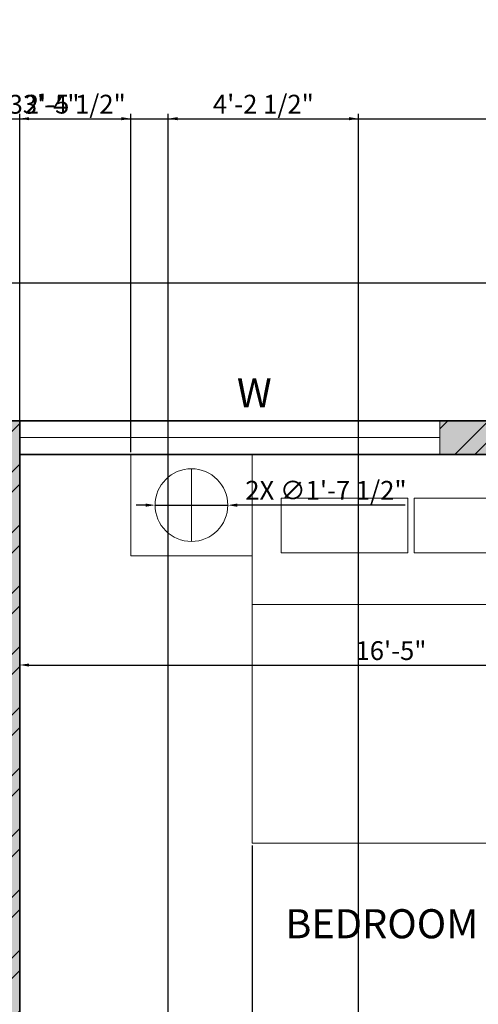
# Model space of a CAD drawing. Units: inches. Extents: x 1804 to 3296, y 909 to 2477.
# Tile 19 of 31: x 2119 to 2241, y 1638 to 1900. Entities that reach past the tile are written whole.
import ezdxf

# ---------------------------------------------------------------- set-up
doc = ezdxf.new("R2010")
doc.units = ezdxf.units.IN
for name, color, linetype, lineweight in [('A-ANNO-DIMS', 2, 'Continuous', 18), ('A-ANNO-TTLB', 156, 'Continuous', 35), ('A-AREA-IDEN', 190, 'Continuous', 18), ('A-WALL-PATT', 10, 'Continuous', 13), ('C-PROP', 7, 'Continuous', 25), ('FUR', 100, 'Continuous', 18), ('TEXT', 190, 'Continuous', 18), ('WALL', 10, 'Continuous', 35), ('WIND', 130, 'Continuous', 18)]:
    doc.layers.add(name, color=color, linetype=linetype, lineweight=lineweight)
doc.styles.get("Standard").update_dxf_attribs({"font": 'arial.ttf'})
doc.dimstyles.new('ISO-25', dxfattribs={"dimtxt": 5, "dimasz": 2.5, "dimexe": 1.25, "dimexo": 0.625, "dimtad": 1, "dimdec": 0, "dimlunit": 4, "dimtxsty": 'Standard', "dimcen": 2.5, "dimadec": 0, "dimazin": 0, "dimtfac": 1, "dimtdec": 0, "dimtmove": 0, "dimatfit": 3, "dimfxl": 1, "dimarcsym": 0})
pattern_1 = [(45, (0, 196.207), (-8.08223, 8.08223), []), (45, (5.388, 196.207), (-8.08223, 8.08223), [])]

# ---------------------------------------------------------------- blocks, each defined once
blk = doc.blocks.new('*D10')
at = {"layer": 'A-ANNO-DIMS', "color": 0, "lineweight": -2, "transparency": 16777216}
for p, q in [((2119.08, 1783.75), (2119.08, 1727.15)), ((2316.54, 1783.75), (2316.54, 1727.15)), ((2121.58, 1728.4), (2314.04, 1728.4))]:
    blk.add_line(p, q, dxfattribs=at)
at = {"layer": 'A-ANNO-DIMS', "color": 0, "lineweight": 100, "transparency": 16777216}
for points in [[(2121.58, 1728.81), (2121.58, 1727.98), (2119.08, 1728.4)], [(2314.04, 1728.81), (2314.04, 1727.98), (2316.54, 1728.4)]]:
    blk.add_solid(points, dxfattribs=at)
at = {"layer": 'Defpoints', "color": 0, "lineweight": 100, "transparency": 16777216}
for p in [(2119.08, 1784.38), (2316.54, 1784.38), (2316.54, 1728.4)]:
    blk.add_point(p, dxfattribs=at)
at = {"layer": 'A-ANNO-DIMS', "color": 0, "transparency": 16777216, "insert": (2217.81, 1731.58), "char_height": 5, "attachment_point": 5}
blk.add_mtext('16\'-5"', dxfattribs=at)
blk = doc.blocks.new('WINDOW-PLAN-112IN')
blk.add_line((0, 4.5), (111.7, 4.5))
blk.add_lwpolyline([(0, 0), (111.7, 0), (111.7, 9), (0, 9)], close=True)
blk = doc.blocks.new('NIGHTSTAND-WITH-LAMP')
for p, q in [((16.12, 3.78), (16.12, 23.13)), ((6.45, 13.46), (25.79, 13.46))]:
    blk.add_line(p, q)
blk.add_lwpolyline([(32.24, 26.91), (0, 26.91), (0, 0), (32.24, 0)], close=True)
blk.add_circle((16.12, 13.46), 9.67)
blk = doc.blocks.new('*D51')
at = {"layer": 'A-ANNO-DIMS', "color": 0, "lineweight": -2, "transparency": 16777216}
for p, q in [((1925.58, 1830.66), (1925.58, 1874.99)), ((1928.08, 1873.74), (2323.04, 1873.74)), ((2325.54, 1830.66), (2325.54, 1874.99))]:
    blk.add_line(p, q, dxfattribs=at)
at = {"layer": 'A-ANNO-DIMS', "color": 0, "lineweight": 100, "transparency": 16777216}
for points in [[(1928.08, 1874.15), (1928.08, 1873.32), (1925.58, 1873.74)], [(2323.04, 1874.15), (2323.04, 1873.32), (2325.54, 1873.74)]]:
    blk.add_solid(points, dxfattribs=at)
at = {"layer": 'Defpoints', "color": 0, "lineweight": 100, "transparency": 16777216}
for p in [(2325.54, 1873.74), (1925.58, 1830.04), (2325.54, 1830.04)]:
    blk.add_point(p, dxfattribs=at)
at = {"layer": 'A-ANNO-DIMS', "color": 0, "transparency": 16777216, "insert": (2125.56, 1876.92), "char_height": 5, "attachment_point": 5}
blk.add_mtext('33\'-4"', dxfattribs=at)
blk = doc.blocks.new('*D56')
at = {"layer": 'A-ANNO-DIMS', "color": 0, "lineweight": -2, "transparency": 16777216}
for p, q in [((2180.87, 1680.42), (2180.87, 975.89)), ((2268, 1680.42), (2268, 975.89)), ((2183.37, 977.14), (2265.5, 977.14))]:
    blk.add_line(p, q, dxfattribs=at)
at = {"layer": 'A-ANNO-DIMS', "color": 0, "lineweight": 100, "transparency": 16777216}
for points in [[(2183.37, 977.56), (2183.37, 976.72), (2180.87, 977.14)], [(2265.5, 977.56), (2265.5, 976.72), (2268, 977.14)]]:
    blk.add_solid(points, dxfattribs=at)
at = {"layer": 'Defpoints', "color": 0, "lineweight": 100, "transparency": 16777216}
for p in [(2180.87, 1681.04), (2268, 1681.04), (2268, 977.14)]:
    blk.add_point(p, dxfattribs=at)
at = {"layer": 'A-ANNO-DIMS', "color": 0, "transparency": 16777216, "insert": (2224.44, 980.32), "char_height": 5, "attachment_point": 5}
blk.add_mtext('7\'-3"', dxfattribs=at)
blk = doc.blocks.new('*D58')
at = {"layer": 'A-ANNO-DIMS', "color": 0, "lineweight": -2, "transparency": 16777216}
for p, q in [((2119.08, 1785), (2119.08, 1874.99)), ((2121.58, 1873.74), (2146.13, 1873.74)), ((2148.63, 1785), (2148.63, 1874.99))]:
    blk.add_line(p, q, dxfattribs=at)
at = {"layer": 'A-ANNO-DIMS', "color": 0, "lineweight": 100, "transparency": 16777216}
for points in [[(2121.58, 1874.15), (2121.58, 1873.32), (2119.08, 1873.74)], [(2146.13, 1874.15), (2146.13, 1873.32), (2148.63, 1873.74)]]:
    blk.add_solid(points, dxfattribs=at)
at = {"layer": 'Defpoints', "color": 0, "lineweight": 100, "transparency": 16777216}
for p in [(2148.63, 1873.74), (2119.08, 1784.38), (2148.63, 1784.38)]:
    blk.add_point(p, dxfattribs=at)
at = {"layer": 'A-ANNO-DIMS', "color": 0, "transparency": 16777216, "insert": (2133.86, 1876.95), "char_height": 5, "attachment_point": 5}
blk.add_mtext('2\'-5 1/2"', dxfattribs=at)
blk = doc.blocks.new('*D71')
at = {"layer": 'A-ANNO-DIMS', "color": 0, "lineweight": -2, "transparency": 16777216}
for p, q in [((2158.58, 1272.26), (2158.58, 1874.99)), ((2161.08, 1873.74), (2206.69, 1873.74)), ((2209.19, 1272.26), (2209.19, 1874.99))]:
    blk.add_line(p, q, dxfattribs=at)
at = {"layer": 'A-ANNO-DIMS', "color": 0, "lineweight": 100, "transparency": 16777216}
for points in [[(2161.08, 1874.15), (2161.08, 1873.32), (2158.58, 1873.74)], [(2206.69, 1874.15), (2206.69, 1873.32), (2209.19, 1873.74)]]:
    blk.add_solid(points, dxfattribs=at)
at = {"layer": 'Defpoints', "color": 0, "lineweight": 100, "transparency": 16777216}
for p in [(2209.19, 1873.74), (2158.58, 1271.63), (2209.19, 1271.63)]:
    blk.add_point(p, dxfattribs=at)
at = {"layer": 'A-ANNO-DIMS', "color": 0, "transparency": 16777216, "insert": (2183.88, 1876.95), "char_height": 5, "attachment_point": 5}
blk.add_mtext('4\'-2 1/2"', dxfattribs=at)
blk = doc.blocks.new('*D102')
at = {"layer": 'A-ANNO-DIMS', "color": 0, "lineweight": -2, "transparency": 16777216}
for p, q in [((2152.58, 1770.93), (2150.08, 1770.93)), ((2155.08, 1770.93), (2174.42, 1770.92)), ((2221.62, 1770.9), (2176.92, 1770.92))]:
    blk.add_line(p, q, dxfattribs=at)
at = {"layer": 'A-ANNO-DIMS', "color": 0, "lineweight": 100, "transparency": 16777216}
for points in [[(2152.58, 1771.35), (2152.58, 1770.51), (2155.08, 1770.93)], [(2176.92, 1771.34), (2176.92, 1770.5), (2174.42, 1770.92)]]:
    blk.add_solid(points, dxfattribs=at)
at = {"layer": 'Defpoints', "color": 0, "lineweight": 100, "transparency": 16777216}
for p in [(2155.08, 1770.93), (2174.42, 1770.92)]:
    blk.add_point(p, dxfattribs=at)
at = {"layer": 'A-ANNO-DIMS', "color": 0, "transparency": 16777216, "insert": (2200.52, 1774.23), "char_height": 5, "attachment_point": 5, "rotation": 359.9776}
blk.add_mtext('2X ∅1\'-7 1/2"', dxfattribs=at)

msp = doc.modelspace()

# ---------------------------------------------------------------- hatches: boundary and pattern name
at = {"layer": 'A-ANNO-TTLB'}
h = msp.add_hatch(color=256, dxfattribs=at)
h.dxf.hatch_style = 1
h.paths.add_polyline_path([(3294.53, 2476.54), (1803.79, 2476.54), (1805.43, 909.47), (3296.17, 909.47)])
h.paths.add_polyline_path([(1811, 914.33), (1812.79, 2467.54), (3285.53, 2467.54), (3283.74, 914.33)], flags=16)
h.paths.add_polyline_path([(1925.58, 1062.77), (1925.58, 1138.07), (1925.58, 1539.88), (1925.58, 1793.38), (1925.58, 1830.04), (2325.54, 1830.04), (2325.54, 1793.38), (2325.54, 1586.42), (2325.54, 1138.07), (2325.54, 1062.77)], flags=0)
h.paths.add_polyline_path([(1997.22, 1029.4), (2008.85, 1037.96), (2008.85, 1020.84)], flags=0)
h.paths.add_polyline_path([(1934.58, 1138.07), (1934.58, 1147.07), (2078.77, 1147.07), (2078.77, 1138.07), (2060.94, 1138.07)], flags=0)
h.paths.add_polyline_path([(1944.35, 1138.07), (1944.35, 1147.07), (2056.05, 1147.07), (2056.05, 1138.07)], flags=0)
h.paths.add_polyline_path([(2222.24, 1037.96), (2233.87, 1029.4), (2222.24, 1020.84)], flags=0)
h.paths.add_polyline_path([(2061.94, 1139.07), (2061.94, 1146.07), (2077.77, 1146.07), (2077.77, 1139.07)], flags=0)
h.paths.add_polyline_path([(2149.58, 1138.07), (2149.58, 1269.44), (2158.58, 1269.44), (2158.58, 1326.69), (2149.58, 1326.69), (2149.58, 1340.94), (2139.6, 1340.94), (2139.6, 1434.25), (2149.58, 1434.25), (2149.58, 1447.36), (2158.58, 1447.36), (2158.58, 1423.87), (2158.58, 1408.06), (2198.46, 1408.06), (2198.46, 1412.56), (2282.65, 1412.56), (2282.65, 1465.94), (2316.54, 1465.94), (2316.54, 1590.92), (2192.86, 1590.92), (2192.86, 1595.3), (2291.17, 1595.3), (2291.17, 1590.92), (2316.54, 1590.92), (2316.54, 1784.38), (2300.24, 1784.38), (2300.24, 1757.47), (2268, 1757.47), (2268, 1681.04), (2180.87, 1681.04), (2180.87, 1757.47), (2148.63, 1757.47), (2148.63, 1784.38), (2119.08, 1784.38), (2119.08, 1585.58), (2114.58, 1585.58), (2114.58, 1784.38), (2064.11, 1784.38), (2046.28, 1784.38), (2046.28, 1760.38), (1958.58, 1760.38), (1958.58, 1664.38), (1934.58, 1664.38), (1934.58, 1784.38), (1934.58, 1793.38), (2046.28, 1793.38), (2064.11, 1793.38), (2119.08, 1793.38), (2230.78, 1793.38), (2230.78, 1784.38), (2268, 1784.38), (2300.24, 1784.38), (2316.54, 1784.38), (2316.54, 1590.92), (2316.54, 1373.73), (2316.54, 1138.07)], flags=0)
h.paths.add_polyline_path([(2209.19, 1166.63), (2209.19, 1175.63), (2158.58, 1175.63), (2209.19, 1223.63), (2209.19, 1231.63), (2183.88, 1231.63), (2183.88, 1301.66), (2242.59, 1301.66), (2242.59, 1326.69), (2316.54, 1326.69), (2272.59, 1271.63), (2272.59, 1223.63), (2316.54, 1175.63), (2272.59, 1175.63), (2272.59, 1166.63)], flags=0)
h.paths.add_polyline_path([(1947.77, 1345.22), (1947.77, 1457.48), (1991.2, 1457.48), (1991.2, 1451.7), (1991.2, 1352.18), (1991.2, 1345.22)], flags=0)
h.paths.add_polyline_path([(2209.19, 1271.63), (2262.59, 1271.63), (2262.59, 1311.85), (2272.59, 1301.66), (2272.59, 1271.63), (2269.92, 1269.63), (2270.59, 1269.63), (2270.59, 1225.63), (2211.19, 1225.63), (2211.19, 1269.63), (2211.86, 1269.63)], flags=0)
h.paths.add_polyline_path([(2000.34, 1378.21), (2000.34, 1429.71), (2025.22, 1429.71), (2025.22, 1378.21)], flags=0)
h.paths.add_polyline_path([(2001.34, 1379.21), (2001.34, 1428.71), (2024.22, 1428.71), (2024.22, 1379.21)], flags=0)
h.paths.add_polyline_path([(2012.34, 1390.21), (2012.34, 1417.71), (2013.22, 1417.71), (2013.22, 1390.21)], flags=0)
h.paths.add_polyline_path([(2237.56, 1331.19), (2237.56, 1340.18), (2238.62, 1340.18), (2238.62, 1386.84), (2241.04, 1386.84), (2242.06, 1386.84), (2242.06, 1408.06), (2316.54, 1331.19)], flags=0)
h.paths.add_polyline_path([(1953.73, 1464.35), (1953.73, 1498.59), (1981.74, 1498.59), (1981.74, 1464.35)], flags=0)
h.paths.add_polyline_path([(1987.63, 1462.08), (1987.63, 1500.95), (2104.07, 1500.95), (2104.07, 1462.08), (2099.27, 1462.08), (1993.6, 1462.08)], flags=0)
h.paths.add_polyline_path([(1956.06, 1481.47, -1), (1979.41, 1481.47, -1)], flags=0)
edge = h.paths.add_edge_path(flags=0)
edge.add_ellipse((2299.53, 1438.37), major_axis=(0.31, 21.36), ratio=0.670333, start_angle=0, end_angle=360)
h.paths.add_polyline_path([(2297.39, 1438.37, -1), (2301.67, 1438.37, -1)], flags=0)
h.paths.add_polyline_path([(2591.54, 1163.23), (2591.54, 1179.38), (2591.54, 1379.68), (2591.54, 1395.84), (2734.5, 1395.84), (2734.5, 1379.68), (2734.5, 1179.38), (2734.5, 1163.23)], flags=0)
h.paths.add_polyline_path([(2592.54, 1164.23), (2592.54, 1166.23), (2733.5, 1166.23), (2733.5, 1164.23)], flags=0)
h.paths.add_polyline_path([(2592.54, 1180.38), (2592.54, 1378.68), (2733.5, 1378.68), (2733.5, 1180.38)], flags=0)
h.paths.add_polyline_path([(2593.54, 1181.38), (2593.54, 1377.68), (2732.5, 1377.68), (2732.5, 1181.38)], flags=0)
h.paths.add_polyline_path([(2594.54, 1182.38), (2594.54, 1376.68), (2731.5, 1376.68), (2731.5, 1182.38)], flags=0)
h.paths.add_polyline_path([(1936.95, 1697.46), (1936.95, 1736.46), (1955.41, 1736.46), (1955.41, 1697.46)], flags=0)
h.paths.add_polyline_path([(1938.48, 1718.36), (1938.48, 1734.92), (1953.65, 1734.92), (1953.65, 1718.36)], flags=0)
h.paths.add_polyline_path([(1944.75, 1726.64, -1), (1947.37, 1726.64, -1)], flags=0)
h.paths.add_polyline_path([(2592.54, 1394.84), (2733.5, 1394.84), (2733.5, 1392.84), (2592.54, 1392.84)], flags=0)
h.paths.add_polyline_path([(1976.61, 1762.5), (1976.61, 1781.44), (2012.79, 1781.44), (2012.79, 1762.5)], flags=0)
h.paths.add_polyline_path([(1979.57, 1771.97, -1), (1991.39, 1771.97, -1)], flags=0)
h.paths.add_polyline_path([(1995.36, 1771.97, -1), (2007.18, 1771.97, -1)], flags=0)
h.paths.add_polyline_path([(2251.51, 1744.53), (2268, 1730.05), (2251.51, 1730.05)], flags=0)
h.paths.add_polyline_path([(2047.28, 1785.38), (2047.28, 1792.38), (2063.11, 1792.38), (2063.11, 1785.38)], flags=0)
h.paths.add_polyline_path([(2155.08, 1770.92, -1), (2174.42, 1770.92, -1)], flags=0)
h.paths.add_polyline_path([(2188.59, 1758.27), (2188.59, 1772.81), (2222.3, 1772.81), (2222.3, 1758.27)], flags=0)
h.paths.add_polyline_path([(2223.97, 1758.27), (2223.97, 1772.81), (2257.68, 1772.81), (2257.68, 1758.27)], flags=0)
h.paths.add_polyline_path([(2274.45, 1770.92, -1), (2293.8, 1770.92, -1)], flags=0)
h.paths.add_polyline_path([(2591.54, 1582.09), (2591.54, 1782.39), (2734.5, 1782.39), (2734.5, 1582.09)], flags=0)
h.paths.add_polyline_path([(2592.54, 1583.09), (2592.54, 1781.39), (2733.5, 1781.39), (2733.5, 1583.09)], flags=0)
h.paths.add_polyline_path([(2593.54, 1584.09), (2593.54, 1780.39), (2732.5, 1780.39), (2732.5, 1584.09)], flags=0)
h.paths.add_polyline_path([(2594.54, 1585.09), (2594.54, 1779.39), (2731.5, 1779.39), (2731.5, 1585.09)], flags=0)
h.paths.add_polyline_path([(1922.17, 1978.79), (1922.17, 2295.08), (1922.17, 2296.08), (2115.67, 2296.08), (2115.67, 2384.31), (2115.67, 2385.31), (2322.12, 2385.31), (2323.12, 2385.31), (2323.12, 1979.79), (2323.12, 1978.79), (1923.17, 1978.79)], flags=0)
h.paths.add_polyline_path([(1922.17, 1978.79), (1922.17, 2051.31), (1922.17, 2214.86), (1922.17, 2296.08), (2115.67, 2296.08), (2115.67, 2385.31), (2323.12, 2385.31), (2323.12, 2280.42), (2323.12, 1978.79), (2115.67, 1978.79)], flags=0)
h.paths.add_polyline_path([(1923.17, 1979.79), (1923.17, 2050.31), (2115.67, 2050.31), (2115.67, 2051.31), (1923.17, 2051.31), (1923.17, 2213.86), (1923.17, 2214.86), (1923.17, 2295.08), (1990.02, 2295.08), (1990.02, 2214.86), (1991.02, 2214.86), (1991.02, 2295.08), (2115.67, 2295.08), (2115.67, 1979.79), (2116.67, 1979.79), (2116.67, 2304.18), (2116.67, 2384.31), (2322.12, 2384.31), (2322.12, 2280.42), (2322.12, 1979.79), (2115.67, 1979.79)], flags=0)
h.paths.add_polyline_path([(2972.46, 1192.5), (2972.46, 1196.92), (2995.47, 1196.92), (2995.47, 1255.47), (2995.09, 1255.47), (2987.42, 1249.39), (2980.08, 1255.47), (2978.05, 1255.47), (2978.05, 1257.24), (2995.47, 1257.24), (2995.47, 1261.58), (3015.37, 1261.58), (3015.37, 1333.28), (3015.37, 1414.4), (3032.82, 1414.4), (3032.82, 1333.28), (3032.82, 1261.58), (3052.66, 1261.58), (3052.66, 1255.47), (3079.86, 1255.47), (3078.72, 1254.57), (3081.47, 1252.29), (3078.56, 1249.99), (3075.81, 1252.26), (3072.57, 1249.69), (3070.36, 1251.52), (3067.67, 1249.39), (3060.34, 1255.47), (3052.66, 1255.47), (3052.66, 1196.92), (3054.58, 1196.92), (3074, 1196.92), (3074, 1192.5), (3052.66, 1192.5), (2995.47, 1192.5)], flags=0)
h.paths.add_polyline_path([(2490.75, 1979.27), (2490.75, 1980.27), (2596.87, 1980.27), (2596.87, 2051.8), (2596.87, 2052.8), (2596.87, 2216.35), (2596.87, 2297.57), (2717.32, 2297.57), (2710.57, 2305.62), (2724.07, 2305.62), (2717.32, 2297.57), (2782.37, 2297.57), (2782.37, 2395.8), (3006.82, 2395.8), (3006.82, 1981.27), (3093.73, 1981.27), (3093.73, 1980.27), (3047.51, 1980.27), (3046.37, 1979.37), (3049.11, 1977.1), (3046.2, 1974.79), (3043.46, 1977.07), (3040.21, 1974.49), (3038, 1976.32), (3035.32, 1974.2), (3027.98, 1980.27), (2871.83, 1980.27), (2871.83, 1981.27), (2791.37, 1981.27), (2791.37, 2050.8), (2597.87, 2050.8), (2597.87, 1980.27), (2597.87, 1979.27), (2546.27, 1979.27), (2545.12, 1978.37), (2547.87, 1976.1), (2544.96, 1973.79), (2542.22, 1976.07), (2538.97, 1973.49), (2536.76, 1975.32), (2534.07, 1973.2), (2526.74, 1979.27)], flags=0)
h.paths.add_polyline_path([(2597.87, 2051.8), (2606.87, 2051.8), (2606.87, 2258.39), (2597.87, 2258.39), (2597.87, 2296.57), (2606.87, 2296.57), (2606.87, 2262.39), (2782.37, 2262.39), (2782.37, 2296.57), (2790.37, 2296.57), (2790.37, 2262.39), (2791.37, 2262.39), (2791.37, 2305.67), (2791.37, 2385.8), (2996.82, 2385.8), (2996.82, 2339.85), (3006.82, 2339.85), (3006.82, 2250.12), (2997.82, 2250.12), (2997.82, 1981.27), (2996.82, 1981.27), (2872.83, 1981.27), (2872.83, 1991.8), (2871.83, 1991.8), (2871.83, 2050.8), (2790.37, 2050.8), (2597.87, 2050.8)], flags=0)
h.paths.add_polyline_path([(2179.93, 2153.92), (2179.93, 2353.97), (2259.98, 2353.97), (2259.98, 2153.92)], flags=0)
h.paths.add_polyline_path([(2180.93, 2154.92), (2180.93, 2352.97), (2258.98, 2352.97), (2258.98, 2154.92)], flags=0)
h.paths.add_polyline_path([(2960.87, 1608.49), (2960.87, 1753.62), (3070.9, 1753.62), (3070.9, 1608.49)], flags=0)
h.paths.add_polyline_path([(2961.87, 1609.49), (2961.87, 1752.62), (3069.9, 1752.62), (3069.9, 1609.49)], flags=0)
h.paths.add_polyline_path([(2962.87, 1610.49), (2962.87, 1751.62), (3068.9, 1751.62), (3068.9, 1610.49)], flags=0)
h.paths.add_polyline_path([(2963.87, 1611.49), (2963.87, 1750.62), (3067.9, 1750.62), (3067.9, 1611.49)], flags=0)
h.paths.add_polyline_path([(2782.37, 2051.8), (2782.37, 2216.32), (2791.37, 2216.32), (2791.37, 2051.8), (2872.83, 2051.8), (2872.83, 2068.56), (2884.67, 2068.56), (2884.67, 2085.33), (2896.51, 2085.33), (2896.51, 2102.09), (2908.36, 2102.09), (2908.36, 2118.85), (2920.2, 2118.85), (2920.2, 2135.62), (2932.05, 2135.62), (2932.05, 2145.3), (2925.08, 2145.3), (2925.08, 2203.2), (2996.82, 2203.2), (2996.82, 2145.3), (2953.82, 2145.3), (2872.83, 2051.8), (2790.37, 2051.8)], flags=0)
h.paths.add_polyline_path([(2717.32, 2238.65), (2710.57, 2246.7), (2724.07, 2246.7)], flags=0)
h.paths.add_polyline_path([(2003.09, 1122.79), (2017.16, 1122.79), (2017.16, 1138.74), (2003.09, 1138.74)], flags=8)
h.paths.add_polyline_path([(2174.76, 1792.72), (2188.83, 1792.72), (2188.83, 1808.66), (2174.76, 1808.66)], flags=8)
h.paths.add_polyline_path([(1987.95, 1792.51), (2002.02, 1792.51), (2002.02, 1808.45), (1987.95, 1808.45)], flags=8)
h.paths.add_polyline_path([(2148.79, 1289.26), (2160.46, 1289.26), (2160.46, 1305.2), (2148.79, 1305.2)], flags=8)
h.paths.add_polyline_path([(2115.36, 1133.57), (2127.04, 1133.57), (2127.04, 1149.51), (2115.36, 1149.51)], flags=8)
h.paths.add_polyline_path([(2237.58, 1421.48), (2249.25, 1421.48), (2249.25, 1437.43), (2237.58, 1437.43)], flags=8)
h.paths.add_polyline_path([(2134.99, 1584.32), (2146.66, 1584.32), (2146.66, 1600.26), (2134.99, 1600.26)], flags=8)
h.paths.add_polyline_path([(2101.95, 1557.31), (2113.62, 1557.31), (2113.62, 1573.25), (2101.95, 1573.25)], flags=8)
h.paths.add_polyline_path([(2937.85, 1156.77), (3120.41, 1156.77), (3120.41, 1185.72), (2937.85, 1185.72)], flags=8)
h.paths.add_polyline_path([(2980.71, 1786.71), (3050.06, 1786.71), (3050.06, 1802.66), (2980.71, 1802.66)], flags=8)
h.paths.add_polyline_path([(2869.28, 1661.96), (2938.62, 1661.96), (2938.62, 1690.8), (2869.28, 1690.8)], flags=8)
h.paths.add_polyline_path([(3092.27, 1674.86), (3161.62, 1674.86), (3161.62, 1690.8), (3092.27, 1690.8)], flags=8)
h.paths.add_polyline_path([(2980.71, 1674.86), (3050.06, 1674.86), (3050.06, 1690.8), (2980.71, 1690.8)], flags=8)
h.paths.add_polyline_path([(2649.07, 1678.23), (2674.53, 1678.23), (2674.53, 1714.76), (2649.07, 1714.76)], flags=8)
h.paths.add_polyline_path([(2530.84, 1981.63), (2549.13, 1981.63), (2549.13, 1997.57), (2530.84, 1997.57)], flags=8)
h.paths.add_polyline_path([(3031.29, 1981.77), (3049.58, 1981.77), (3049.58, 1997.71), (3031.29, 1997.71)], flags=8)
h.paths.add_polyline_path([(2715.38, 1911.9), (2851.54, 1911.9), (2851.54, 1940.85), (2715.38, 1940.85)], flags=8)
h.paths.add_polyline_path([(2015.23, 1927.36), (2205.42, 1927.36), (2205.42, 1956.3), (2015.23, 1956.3)], flags=8)
h.paths.add_polyline_path([(2671.84, 2057.84), (2702.75, 2057.84), (2702.75, 2073.79), (2671.84, 2073.79)], flags=8)
h.paths.add_polyline_path([(2678.5, 2316.52), (2765.26, 2316.52), (2765.26, 2332.46), (2678.5, 2332.46)], flags=8)
h.paths.add_polyline_path([(2678.48, 2271.96), (2736.41, 2271.96), (2736.41, 2287.9), (2678.48, 2287.9)], flags=8)
h.paths.add_polyline_path([(2019.2, 972.79), (2243.21, 972.79), (2243.21, 1001.74), (2019.2, 1001.74)], flags=8)
h.paths.add_polyline_path([(2097.06, 1021.56), (2132.16, 1021.56), (2132.16, 1037.51), (2097.06, 1037.51)], flags=8)
h.paths.add_polyline_path([(2182.47, 1360.48), (2207.35, 1360.48), (2207.35, 1376.42), (2182.47, 1376.42)], flags=8)
h.paths.add_polyline_path([(2261.12, 1361.77), (2295.01, 1361.77), (2295.01, 1377.71), (2261.12, 1377.71)], flags=8)
h.paths.add_polyline_path([(2245.75, 1511.51), (2278.44, 1511.51), (2278.44, 1527.46), (2245.75, 1527.46)], flags=8)
h.paths.add_polyline_path([(1991.16, 1296.29), (2060.51, 1296.29), (2060.51, 1312.23), (1991.16, 1312.23)], flags=8)
h.paths.add_polyline_path([(2187, 1651.35), (2246.71, 1651.35), (2246.71, 1667.29), (2187, 1667.29)], flags=8)
h.paths.add_polyline_path([(1976.49, 1684.81), (2068.63, 1684.81), (2068.63, 1700.76), (1976.49, 1700.76)], flags=8)
at = {"layer": 'A-WALL-PATT'}
h = msp.add_hatch(color=256, dxfattribs=at)
h.dxf.hatch_style = 1
h.paths.add_polyline_path([(2119.08, 1544.38), (1925.58, 1544.38), (1925.58, 1539.88), (2119.08, 1539.88)])
h.paths.add_polyline_path([(2119.08, 1545.58), (2114.58, 1545.58), (2114.58, 1544.38), (2119.08, 1544.38)])
h.paths.add_polyline_path([(1965.87, 1658.79), (1965.87, 1679.09), (1955.57, 1679.09), (1955.57, 1658.79)], flags=9)
h.paths.add_polyline_path([(2293.18, 1677.29), (2293.18, 1697.58), (2282.88, 1697.58), (2282.88, 1677.29)], flags=9)
h.paths.add_polyline_path([(2271.13, 1545.23), (2287.53, 1545.23), (2287.53, 1555.53), (2271.13, 1555.53)], flags=9)
h.paths.add_polyline_path([(2303.26, 1488.52), (2303.26, 1508.82), (2292.95, 1508.82), (2292.95, 1488.52)], flags=9)
h.paths.add_polyline_path([(2271.13, 1393.15), (2287.53, 1393.15), (2287.53, 1403.45), (2271.13, 1403.45)], flags=9)
h.paths.add_polyline_path([(2306.48, 1361.45), (2306.48, 1377.86), (2296.18, 1377.86), (2296.18, 1361.45)], flags=9)
h.paths.add_polyline_path([(2174.54, 1361.45), (2174.54, 1377.86), (2164.23, 1377.86), (2164.23, 1361.45)], flags=9)
h.paths.add_polyline_path([(1968.21, 1333.34), (1968.21, 1353.64), (1957.91, 1353.64), (1957.91, 1333.34)], flags=9)
h.paths.add_polyline_path([(2003.09, 1122.79), (2017.16, 1122.79), (2017.16, 1138.74), (2003.09, 1138.74)], flags=9)
h.paths.add_polyline_path([(2174.76, 1792.72), (2188.83, 1792.72), (2188.83, 1808.66), (2174.76, 1808.66)], flags=9)
h.paths.add_polyline_path([(1987.95, 1792.51), (2002.02, 1792.51), (2002.02, 1808.45), (1987.95, 1808.45)], flags=9)
h.paths.add_polyline_path([(2148.79, 1289.26), (2160.46, 1289.26), (2160.46, 1305.2), (2148.79, 1305.2)], flags=9)
h.paths.add_polyline_path([(2115.36, 1133.57), (2127.04, 1133.57), (2127.04, 1149.51), (2115.36, 1149.51)], flags=9)
h.paths.add_polyline_path([(2237.58, 1421.48), (2249.25, 1421.48), (2249.25, 1437.43), (2237.58, 1437.43)], flags=9)
h.paths.add_polyline_path([(2134.99, 1584.32), (2146.66, 1584.32), (2146.66, 1600.26), (2134.99, 1600.26)], flags=9)
h.paths.add_polyline_path([(2101.95, 1557.31), (2113.62, 1557.31), (2113.62, 1573.25), (2101.95, 1573.25)], flags=9)
h.paths.add_polyline_path([(2937.85, 1156.77), (3120.41, 1156.77), (3120.41, 1185.72), (2937.85, 1185.72)], flags=9)
h.paths.add_polyline_path([(2980.71, 1786.71), (3050.06, 1786.71), (3050.06, 1802.66), (2980.71, 1802.66)], flags=9)
h.paths.add_polyline_path([(2869.28, 1661.96), (2938.62, 1661.96), (2938.62, 1690.8), (2869.28, 1690.8)], flags=9)
h.paths.add_polyline_path([(3092.27, 1674.86), (3161.62, 1674.86), (3161.62, 1690.8), (3092.27, 1690.8)], flags=9)
h.paths.add_polyline_path([(2980.71, 1674.86), (3050.06, 1674.86), (3050.06, 1690.8), (2980.71, 1690.8)], flags=9)
h.paths.add_polyline_path([(2649.07, 1678.23), (2674.53, 1678.23), (2674.53, 1714.76), (2649.07, 1714.76)], flags=9)
h.paths.add_polyline_path([(2530.84, 1981.63), (2549.13, 1981.63), (2549.13, 1997.57), (2530.84, 1997.57)], flags=9)
h.paths.add_polyline_path([(3031.29, 1981.77), (3049.58, 1981.77), (3049.58, 1997.71), (3031.29, 1997.71)], flags=9)
h.paths.add_polyline_path([(2715.38, 1911.9), (2851.54, 1911.9), (2851.54, 1940.85), (2715.38, 1940.85)], flags=9)
h.paths.add_polyline_path([(2015.23, 1927.36), (2205.42, 1927.36), (2205.42, 1956.3), (2015.23, 1956.3)], flags=9)
h.paths.add_polyline_path([(2671.84, 2057.84), (2702.75, 2057.84), (2702.75, 2073.79), (2671.84, 2073.79)], flags=9)
h.paths.add_polyline_path([(2678.5, 2316.52), (2765.26, 2316.52), (2765.26, 2332.46), (2678.5, 2332.46)], flags=9)
h.paths.add_polyline_path([(2678.48, 2271.96), (2736.41, 2271.96), (2736.41, 2287.9), (2678.48, 2287.9)], flags=9)
h.paths.add_polyline_path([(2019.2, 972.79), (2243.21, 972.79), (2243.21, 1001.74), (2019.2, 1001.74)], flags=9)
h.paths.add_polyline_path([(2097.06, 1021.56), (2132.16, 1021.56), (2132.16, 1037.51), (2097.06, 1037.51)], flags=9)
h.paths.add_polyline_path([(2182.47, 1360.48), (2207.35, 1360.48), (2207.35, 1376.42), (2182.47, 1376.42)], flags=9)
h.paths.add_polyline_path([(2261.12, 1361.77), (2295.01, 1361.77), (2295.01, 1377.71), (2261.12, 1377.71)], flags=9)
h.paths.add_polyline_path([(2245.75, 1511.51), (2278.44, 1511.51), (2278.44, 1527.46), (2245.75, 1527.46)], flags=9)
h.paths.add_polyline_path([(1991.16, 1296.29), (2060.51, 1296.29), (2060.51, 1312.23), (1991.16, 1312.23)], flags=9)
h.paths.add_polyline_path([(2187, 1651.35), (2246.71, 1651.35), (2246.71, 1667.29), (2187, 1667.29)], flags=9)
h.paths.add_polyline_path([(1976.49, 1684.81), (2068.63, 1684.81), (2068.63, 1700.76), (1976.49, 1700.76)], flags=9)
h = msp.add_hatch(color=256, dxfattribs=at)
h.dxf.hatch_style = 1
h.paths.add_polyline_path([(2149.58, 1147.07), (2141.21, 1147.07), (2141.21, 1144.07), (2141.21, 1138.07), (2149.58, 1138.07)])
h.paths.add_polyline_path([(2101.21, 1144.07, -0.01877), (2101.32, 1147.07), (2078.77, 1147.07), (2078.77, 1138.07), (2101.21, 1138.07)])
h.paths.add_polyline_path([(2060.94, 1147.07), (2056.05, 1147.07), (2056.05, 1138.07), (2060.94, 1138.07)])
h.paths.add_polyline_path([(1944.35, 1147.07), (1934.58, 1147.07), (1934.58, 1138.07), (1944.35, 1138.07)])
h.paths.add_polyline_path([(2158.58, 1269.44), (2149.58, 1269.44), (2149.58, 1138.07), (2158.58, 1138.07)])
h.paths.add_polyline_path([(2003.09, 1122.79), (2017.16, 1122.79), (2017.16, 1138.74), (2003.09, 1138.74)], flags=9)
h.paths.add_polyline_path([(2174.76, 1792.72), (2188.83, 1792.72), (2188.83, 1808.66), (2174.76, 1808.66)], flags=9)
h.paths.add_polyline_path([(1987.95, 1792.51), (2002.02, 1792.51), (2002.02, 1808.45), (1987.95, 1808.45)], flags=9)
h.paths.add_polyline_path([(2148.79, 1289.26), (2160.46, 1289.26), (2160.46, 1305.2), (2148.79, 1305.2)], flags=9)
h.paths.add_polyline_path([(2115.36, 1133.57), (2127.04, 1133.57), (2127.04, 1149.51), (2115.36, 1149.51)], flags=9)
h.paths.add_polyline_path([(2237.58, 1421.48), (2249.25, 1421.48), (2249.25, 1437.43), (2237.58, 1437.43)], flags=9)
h.paths.add_polyline_path([(2134.99, 1584.32), (2146.66, 1584.32), (2146.66, 1600.26), (2134.99, 1600.26)], flags=9)
h.paths.add_polyline_path([(2101.95, 1557.31), (2113.62, 1557.31), (2113.62, 1573.25), (2101.95, 1573.25)], flags=9)
h.paths.add_polyline_path([(2937.85, 1156.77), (3120.41, 1156.77), (3120.41, 1185.72), (2937.85, 1185.72)], flags=9)
h.paths.add_polyline_path([(2980.71, 1786.71), (3050.06, 1786.71), (3050.06, 1802.66), (2980.71, 1802.66)], flags=9)
h.paths.add_polyline_path([(2869.28, 1661.96), (2938.62, 1661.96), (2938.62, 1690.8), (2869.28, 1690.8)], flags=9)
h.paths.add_polyline_path([(3092.27, 1674.86), (3161.62, 1674.86), (3161.62, 1690.8), (3092.27, 1690.8)], flags=9)
h.paths.add_polyline_path([(2980.71, 1674.86), (3050.06, 1674.86), (3050.06, 1690.8), (2980.71, 1690.8)], flags=9)
h.paths.add_polyline_path([(2649.07, 1678.23), (2674.53, 1678.23), (2674.53, 1714.76), (2649.07, 1714.76)], flags=9)
h.paths.add_polyline_path([(2530.84, 1981.63), (2549.13, 1981.63), (2549.13, 1997.57), (2530.84, 1997.57)], flags=9)
h.paths.add_polyline_path([(3031.29, 1981.77), (3049.58, 1981.77), (3049.58, 1997.71), (3031.29, 1997.71)], flags=9)
h.paths.add_polyline_path([(2715.38, 1911.9), (2851.54, 1911.9), (2851.54, 1940.85), (2715.38, 1940.85)], flags=9)
h.paths.add_polyline_path([(2015.23, 1927.36), (2205.42, 1927.36), (2205.42, 1956.3), (2015.23, 1956.3)], flags=9)
h.paths.add_polyline_path([(2671.84, 2057.84), (2702.75, 2057.84), (2702.75, 2073.79), (2671.84, 2073.79)], flags=9)
h.paths.add_polyline_path([(2678.5, 2316.52), (2765.26, 2316.52), (2765.26, 2332.46), (2678.5, 2332.46)], flags=9)
h.paths.add_polyline_path([(2678.48, 2271.96), (2736.41, 2271.96), (2736.41, 2287.9), (2678.48, 2287.9)], flags=9)
h.paths.add_polyline_path([(2019.2, 972.79), (2243.21, 972.79), (2243.21, 1001.74), (2019.2, 1001.74)], flags=9)
h.paths.add_polyline_path([(2097.06, 1021.56), (2132.16, 1021.56), (2132.16, 1037.51), (2097.06, 1037.51)], flags=9)
h.paths.add_polyline_path([(2182.47, 1360.48), (2207.35, 1360.48), (2207.35, 1376.42), (2182.47, 1376.42)], flags=9)
h.paths.add_polyline_path([(2261.12, 1361.77), (2295.01, 1361.77), (2295.01, 1377.71), (2261.12, 1377.71)], flags=9)
h.paths.add_polyline_path([(2245.75, 1511.51), (2278.44, 1511.51), (2278.44, 1527.46), (2245.75, 1527.46)], flags=9)
h.paths.add_polyline_path([(1991.16, 1296.29), (2060.51, 1296.29), (2060.51, 1312.23), (1991.16, 1312.23)], flags=9)
h.paths.add_polyline_path([(2187, 1651.35), (2246.71, 1651.35), (2246.71, 1667.29), (2187, 1667.29)], flags=9)
h.paths.add_polyline_path([(1976.49, 1684.81), (2068.63, 1684.81), (2068.63, 1700.76), (1976.49, 1700.76)], flags=9)
h = msp.add_hatch(color=256, dxfattribs=at)
h.dxf.hatch_style = 1
h.paths.add_polyline_path([(2158.58, 1275.49), (2155.29, 1275.49), (2149.58, 1275.49), (2149.58, 1269.44), (2158.58, 1269.44)])
h.paths.add_polyline_path([(2158.58, 1326.69), (2149.58, 1326.69), (2149.58, 1319.33), (2155.29, 1319.33), (2158.58, 1319.33)])
h.paths.add_polyline_path([(2158.58, 1402.2), (2158.58, 1423.87), (2158.58, 1447.36), (2149.58, 1447.36), (2149.58, 1423.87), (2149.58, 1340.94), (2149.58, 1326.69), (2158.58, 1326.69), (2158.58, 1354.23)])
h.paths.add_polyline_path([(1965.87, 1658.79), (1965.87, 1679.09), (1955.57, 1679.09), (1955.57, 1658.79)], flags=9)
h.paths.add_polyline_path([(2293.18, 1677.29), (2293.18, 1697.58), (2282.88, 1697.58), (2282.88, 1677.29)], flags=9)
h.paths.add_polyline_path([(2271.13, 1545.23), (2287.53, 1545.23), (2287.53, 1555.53), (2271.13, 1555.53)], flags=9)
h.paths.add_polyline_path([(2303.26, 1488.52), (2303.26, 1508.82), (2292.95, 1508.82), (2292.95, 1488.52)], flags=9)
h.paths.add_polyline_path([(2271.13, 1393.15), (2287.53, 1393.15), (2287.53, 1403.45), (2271.13, 1403.45)], flags=9)
h.paths.add_polyline_path([(2306.48, 1361.45), (2306.48, 1377.86), (2296.18, 1377.86), (2296.18, 1361.45)], flags=9)
h.paths.add_polyline_path([(2189.9, 1340.62), (2206.31, 1340.62), (2206.31, 1350.92), (2189.9, 1350.92)], flags=9)
h.paths.add_polyline_path([(2174.54, 1361.45), (2174.54, 1377.86), (2164.23, 1377.86), (2164.23, 1361.45)], flags=9)
h.paths.add_polyline_path([(2304.24, 1240.8), (2304.24, 1261.09), (2293.94, 1261.09), (2293.94, 1240.8)], flags=9)
h.paths.add_polyline_path([(2227.19, 1188.73), (2247.49, 1188.73), (2247.49, 1199.03), (2227.19, 1199.03)], flags=9)
h.paths.add_polyline_path([(2181.93, 1144.21), (2181.93, 1160.62), (2171.63, 1160.62), (2171.63, 1144.21)], flags=9)
h.paths.add_polyline_path([(1968.21, 1333.34), (1968.21, 1353.64), (1957.91, 1353.64), (1957.91, 1333.34)], flags=9)
h.paths.add_polyline_path([(2029.78, 1203.53), (2053.95, 1203.53), (2053.95, 1213.83), (2029.78, 1213.83)], flags=9)
h.paths.add_polyline_path([(2576.51, 1671.88), (2576.51, 1692.17), (2566.21, 1692.17), (2566.21, 1671.88)], flags=9)
h.paths.add_polyline_path([(2566.99, 1269.67), (2566.99, 1289.96), (2556.68, 1289.96), (2556.68, 1269.67)], flags=9)
h.paths.add_polyline_path([(2581.85, 1269.17), (2581.85, 1289.46), (2571.54, 1289.46), (2571.54, 1269.17)], flags=9)
h.paths.add_polyline_path([(2650.71, 1409.75), (2674.89, 1409.75), (2674.89, 1420.05), (2650.71, 1420.05)], flags=9)
h.paths.add_polyline_path([(2003.09, 1122.79), (2017.16, 1122.79), (2017.16, 1138.74), (2003.09, 1138.74)], flags=9)
h.paths.add_polyline_path([(2174.76, 1792.72), (2188.83, 1792.72), (2188.83, 1808.66), (2174.76, 1808.66)], flags=9)
h.paths.add_polyline_path([(1987.95, 1792.51), (2002.02, 1792.51), (2002.02, 1808.45), (1987.95, 1808.45)], flags=9)
h.paths.add_polyline_path([(2148.79, 1289.26), (2160.46, 1289.26), (2160.46, 1305.2), (2148.79, 1305.2)], flags=9)
h.paths.add_polyline_path([(2115.36, 1133.57), (2127.04, 1133.57), (2127.04, 1149.51), (2115.36, 1149.51)], flags=9)
h.paths.add_polyline_path([(2237.58, 1421.48), (2249.25, 1421.48), (2249.25, 1437.43), (2237.58, 1437.43)], flags=9)
h.paths.add_polyline_path([(2134.99, 1584.32), (2146.66, 1584.32), (2146.66, 1600.26), (2134.99, 1600.26)], flags=9)
h.paths.add_polyline_path([(2101.95, 1557.31), (2113.62, 1557.31), (2113.62, 1573.25), (2101.95, 1573.25)], flags=9)
h.paths.add_polyline_path([(2937.85, 1156.77), (3120.41, 1156.77), (3120.41, 1185.72), (2937.85, 1185.72)], flags=9)
h.paths.add_polyline_path([(2980.71, 1786.71), (3050.06, 1786.71), (3050.06, 1802.66), (2980.71, 1802.66)], flags=9)
h.paths.add_polyline_path([(2869.28, 1661.96), (2938.62, 1661.96), (2938.62, 1690.8), (2869.28, 1690.8)], flags=9)
h.paths.add_polyline_path([(3092.27, 1674.86), (3161.62, 1674.86), (3161.62, 1690.8), (3092.27, 1690.8)], flags=9)
h.paths.add_polyline_path([(2980.71, 1674.86), (3050.06, 1674.86), (3050.06, 1690.8), (2980.71, 1690.8)], flags=9)
h.paths.add_polyline_path([(2649.07, 1678.23), (2674.53, 1678.23), (2674.53, 1714.76), (2649.07, 1714.76)], flags=9)
h.paths.add_polyline_path([(2530.84, 1981.63), (2549.13, 1981.63), (2549.13, 1997.57), (2530.84, 1997.57)], flags=9)
h.paths.add_polyline_path([(3031.29, 1981.77), (3049.58, 1981.77), (3049.58, 1997.71), (3031.29, 1997.71)], flags=9)
h.paths.add_polyline_path([(2715.38, 1911.9), (2851.54, 1911.9), (2851.54, 1940.85), (2715.38, 1940.85)], flags=9)
h.paths.add_polyline_path([(2015.23, 1927.36), (2205.42, 1927.36), (2205.42, 1956.3), (2015.23, 1956.3)], flags=9)
h.paths.add_polyline_path([(2671.84, 2057.84), (2702.75, 2057.84), (2702.75, 2073.79), (2671.84, 2073.79)], flags=9)
h.paths.add_polyline_path([(2678.5, 2316.52), (2765.26, 2316.52), (2765.26, 2332.46), (2678.5, 2332.46)], flags=9)
h.paths.add_polyline_path([(2678.48, 2271.96), (2736.41, 2271.96), (2736.41, 2287.9), (2678.48, 2287.9)], flags=9)
h.paths.add_polyline_path([(2019.2, 972.79), (2243.21, 972.79), (2243.21, 1001.74), (2019.2, 1001.74)], flags=9)
h.paths.add_polyline_path([(2097.06, 1021.56), (2132.16, 1021.56), (2132.16, 1037.51), (2097.06, 1037.51)], flags=9)
h.paths.add_polyline_path([(2182.47, 1360.48), (2207.35, 1360.48), (2207.35, 1376.42), (2182.47, 1376.42)], flags=9)
h.paths.add_polyline_path([(2261.12, 1361.77), (2295.01, 1361.77), (2295.01, 1377.71), (2261.12, 1377.71)], flags=9)
h.paths.add_polyline_path([(2245.75, 1511.51), (2278.44, 1511.51), (2278.44, 1527.46), (2245.75, 1527.46)], flags=9)
h.paths.add_polyline_path([(1991.16, 1296.29), (2060.51, 1296.29), (2060.51, 1312.23), (1991.16, 1312.23)], flags=9)
h.paths.add_polyline_path([(2187, 1651.35), (2246.71, 1651.35), (2246.71, 1667.29), (2187, 1667.29)], flags=9)
h.paths.add_polyline_path([(1976.49, 1684.81), (2068.63, 1684.81), (2068.63, 1700.76), (1976.49, 1700.76)], flags=9)
h = msp.add_hatch(dxfattribs=at)
h.set_pattern_fill('ANSI32', color=256, scale=1.2)
h.set_pattern_definition(pattern_1)
h.paths.add_polyline_path([(1934.58, 1784.38), (1934.58, 1793.38), (1925.58, 1793.38), (1925.58, 1539.88), (2119.08, 1539.88), (2119.08, 1545.58), (2114.58, 1545.58), (2114.58, 1544.38), (1934.58, 1544.38)])
h.paths.add_polyline_path([(2114.58, 1793.38), (2064.11, 1793.38), (2064.11, 1784.38), (2114.58, 1784.38)], flags=17)
h.paths.add_polyline_path([(2325.54, 1793.38), (2230.78, 1793.38), (2230.78, 1784.38), (2268, 1784.38), (2300.24, 1784.38), (2316.54, 1784.38), (2316.54, 1590.92), (2316.54, 1586.42), (2325.54, 1586.42)])
h.paths.add_polyline_path([(1944.35, 1147.07), (1934.58, 1147.07), (1934.58, 1138.07), (1944.35, 1138.07)])
h.paths.add_polyline_path([(2101.21, 1144.07, -0.01877), (2101.32, 1147.07), (2078.77, 1147.07), (2078.77, 1138.07), (2101.21, 1138.07)])
h.paths.add_polyline_path([(1934.58, 1539.88), (1925.58, 1539.88), (1925.58, 1138.07), (1934.58, 1138.07), (1934.58, 1147.07)])
h.paths.add_polyline_path([(2325.54, 1586.42), (2316.54, 1586.42), (2316.54, 1373.73), (2316.54, 1138.07), (2325.54, 1138.07), (2325.54, 1228.97)])
h.paths.add_polyline_path([(2158.58, 1423.87), (2158.58, 1447.36), (2149.58, 1447.36), (2149.58, 1423.87), (2149.58, 1340.94), (2149.58, 1326.69), (2158.58, 1326.69), (2158.58, 1354.23), (2158.58, 1402.2)])
h.paths.add_polyline_path([(2316.54, 1412.56), (2282.65, 1412.56), (2273.09, 1412.56), (2273.09, 1408.06), (2316.54, 1408.06)])
h.paths.add_polyline_path([(2273.09, 1412.56), (2242.06, 1412.56), (2242.06, 1408.06), (2273.09, 1408.06)])
h.paths.add_polyline_path([(2237.56, 1412.56), (2198.46, 1412.56), (2198.46, 1408.06), (2237.56, 1408.06)])
h.paths.add_polyline_path([(2242.06, 1408.06), (2237.56, 1408.06), (2237.56, 1386.84), (2242.06, 1386.84)])
h.paths.add_polyline_path([(2242.06, 1412.56), (2237.56, 1412.56), (2237.56, 1408.06), (2242.06, 1408.06)])
h.paths.add_polyline_path([(2158.58, 1269.44), (2149.58, 1269.44), (2149.58, 1138.07), (2158.58, 1138.07)])
h.paths.add_polyline_path([(2149.58, 1147.07), (2141.21, 1147.07), (2141.21, 1144.07), (2141.21, 1138.07), (2149.58, 1138.07)])
h.paths.add_polyline_path([(2272.59, 1175.63), (2209.19, 1175.63), (2209.19, 1166.63), (2272.59, 1166.63)])
h.paths.add_polyline_path([(2237.56, 1446.21), (2242.06, 1446.21), (2242.06, 1586.42), (2237.56, 1586.42)])
h.paths.add_polyline_path([(2242.06, 1414.58), (2237.56, 1414.58), (2237.56, 1412.56), (2242.06, 1412.56)])
h = msp.add_hatch(color=256, dxfattribs=at)
h.dxf.hatch_style = 1
h.paths.add_polyline_path([(2114.58, 1793.38), (2064.11, 1793.38), (2064.11, 1784.38), (2114.58, 1784.38)])
h.paths.add_polyline_path([(2119.08, 1793.38), (2114.58, 1793.38), (2114.58, 1585.58), (2119.08, 1585.58)])
h.paths.add_polyline_path([(2325.54, 1793.38), (2230.78, 1793.38), (2230.78, 1784.38), (2268, 1784.38), (2316.54, 1784.38), (2316.54, 1590.92), (2316.54, 1586.42), (2325.54, 1586.42)])
h.paths.add_polyline_path([(2316.54, 1331.19), (2158.58, 1331.19), (2158.58, 1326.69), (2316.54, 1326.69)])
h.paths.add_polyline_path([(2242.06, 1408.06), (2237.56, 1408.06), (2237.56, 1386.84), (2242.06, 1386.84)])
h.paths.add_polyline_path([(2242.06, 1412.56), (2237.56, 1412.56), (2237.56, 1408.06), (2242.06, 1408.06)])
h.paths.add_polyline_path([(2237.56, 1412.56), (2198.46, 1412.56), (2198.46, 1408.06), (2237.56, 1408.06)])
h.paths.add_polyline_path([(2273.09, 1412.56), (2242.06, 1412.56), (2242.06, 1408.06), (2273.09, 1408.06)])
h.paths.add_polyline_path([(2316.54, 1412.56), (2282.65, 1412.56), (2273.09, 1412.56), (2273.09, 1408.06), (2316.54, 1408.06)])
h.paths.add_polyline_path([(2325.54, 1586.42), (2316.54, 1586.42), (2316.54, 1373.73), (2316.54, 1138.07), (2325.54, 1138.07), (2325.54, 1228.97)])
h.paths.add_polyline_path([(2272.59, 1175.63), (2209.19, 1175.63), (2209.19, 1166.63), (2272.59, 1166.63)])
h = msp.add_hatch(dxfattribs=at)
h.set_pattern_fill('ANSI32', color=256, scale=1.2)
h.set_pattern_definition(pattern_1)
h.paths.add_polyline_path([(2114.58, 1585.58), (2119.08, 1585.58), (2119.08, 1793.38), (2114.58, 1793.38)])

# ---------------------------------------------------------------- linework, layer by layer
at = {"layer": 'C-PROP'}
msp.add_line((1925.58, 1830.04), (2325.54, 1830.04), dxfattribs=at)
at = {"layer": 'FUR'}
msp.add_line((2180.87, 1744.53), (2251.51, 1744.53), dxfattribs=at)
for points in [[(2180.87, 1784.38), (2268, 1784.38), (2268, 1681.04), (2180.87, 1681.04)], [(2188.59, 1772.81), (2222.3, 1772.81), (2222.3, 1758.27), (2188.59, 1758.27)], [(2223.97, 1772.81), (2257.68, 1772.81), (2257.68, 1758.27), (2223.97, 1758.27)]]:
    msp.add_lwpolyline(points, close=True, dxfattribs=at)
at = {"layer": 'WALL'}
for p, q in [((1925.58, 1793.38), (2119.08, 1793.38)), ((2119.08, 1793.38), (2119.08, 1585.58)), ((2119.08, 1793.38), (2325.54, 1793.38)), ((2119.08, 1784.38), (2316.54, 1784.38))]:
    msp.add_line(p, q, dxfattribs=at)
msp.add_lwpolyline([(2114.58, 1585.58), (2119.08, 1585.58), (2119.08, 1793.38), (2114.58, 1793.38)], close=True, dxfattribs=at)

# ---------------------------------------------------------------- block references
at = {"layer": 'FUR'}
msp.add_blockref('NIGHTSTAND-WITH-LAMP', (2148.63, 1757.47), dxfattribs=at)
at = {"layer": 'WIND'}
msp.add_blockref('WINDOW-PLAN-112IN', (2119.08, 1784.38), dxfattribs=at)

# ---------------------------------------------------------------- texts
at = {"layer": 'A-AREA-IDEN', "insert": (2189.72, 1663.44), "char_height": 7.737, "attachment_point": 1}
msp.add_mtext_dynamic_manual_height_columns('BEDROOM', width=163.3261, gutter_width=38.69, heights=[0], dxfattribs=at)
at = {"layer": 'TEXT', "insert": (2176.83, 1804.68), "char_height": 7.74, "attachment_point": 1}
msp.add_mtext_dynamic_manual_height_columns('W', width=163.3261, gutter_width=38.69, heights=[0], dxfattribs=at)

# ---------------------------------------------------------------- dimensions: what is measured, and where the dimension line sits
at = {"layer": 'A-ANNO-DIMS'}
for base, p1, p2, override, picture, middle in [((2148.6296, 1873.7362), (2119.0828, 1784.3796), (2148.6296, 1784.3796), {"dimdec": 1, "dimlfac": 1, "dimrnd": 0, "dimzin": 1, "dimdsep": 46, "dimlunit": 4, "dimfrac": 2}, '*D58', (2133.8562, 1876.9465)), ((2209.19, 1873.74), (2158.58, 1271.63), (2209.19, 1271.63), {"dimdec": 1, "dimlfac": 1, "dimrnd": 0, "dimzin": 1, "dimdsep": 46, "dimlunit": 4, "dimfrac": 2}, '*D71', (2183.88, 1876.95)), ((2325.54, 1873.74), (1925.58, 1830.04), (2325.54, 1830.04), {"dimdec": 1, "dimlfac": 1, "dimrnd": 0, "dimzin": 1, "dimdsep": 46, "dimlunit": 4, "dimfrac": 2}, '*D51', (2125.56, 1876.92)), ((2316.54, 1728.4), (2119.08, 1784.38), (2316.54, 1784.38), {"dimclrd": 0, "dimclre": 0, "dimclrt": 0}, '*D10', (2217.81, 1731.58)), ((2268, 977.14), (2180.87, 1681.04), (2268, 1681.04), {"dimdec": 1, "dimlfac": 1, "dimrnd": 0, "dimzin": 1, "dimdsep": 46, "dimlunit": 4, "dimfrac": 2}, '*D56', (2224.44, 980.32))]:
    dim = msp.add_linear_dim(base=base, p1=p1, p2=p2, dimstyle='ISO-25', override=override, dxfattribs=at)
    dim.commit()
    dim.dimension.update_dxf_attribs({"geometry": picture, "text_midpoint": middle})
dim = msp.add_diameter_dim_2p(p1=(2155.08, 1770.93), p2=(2174.42, 1770.92), text='2X <>', dimstyle='ISO-25', override={"dimdec": 1, "dimlfac": 1, "dimrnd": 0, "dimzin": 1, "dimdsep": 46, "dimlunit": 4, "dimfrac": 2}, dxfattribs=at)
dim.commit()
dim.dimension.update_dxf_attribs({"geometry": '*D102', "text_midpoint": (2200.52, 1770.91)})

doc.saveas('drawing.dxf')
